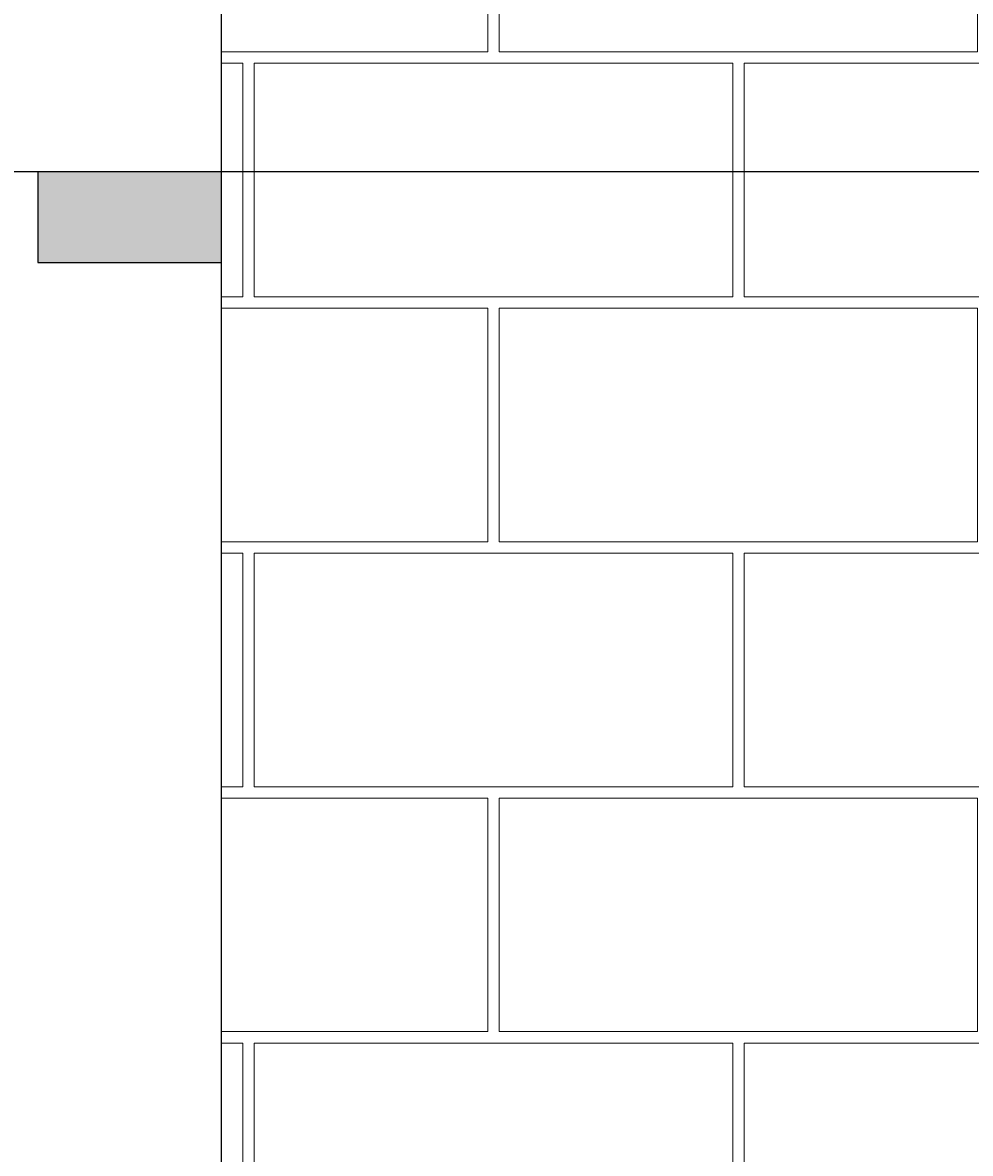
# Model space of a CAD drawing. Units: inches. Extents: x -128 to 854, y -395 to 398.
# Tile 54 of 61: x 405 to 467, y -322 to -248. Entities that reach past the tile are written whole.
import ezdxf

# ---------------------------------------------------------------- set-up
doc = ezdxf.new("R2010")
doc.units = ezdxf.units.IN
doc.header["$MEASUREMENT"] = 0
for name, color, linetype, lineweight in [('A-ANNO-DIMS', 2, 'Continuous', 18), ('A-ELEV', 3, 'Continuous', 25), ('A-ELEV-PATT', 8, 'Continuous', 13)]:
    doc.layers.add(name, color=color, linetype=linetype, lineweight=lineweight)
doc.styles.get("Standard").update_dxf_attribs({"font": 'arial.ttf'})
doc.dimstyles.get("Standard").update_dxf_attribs({"dimtxt": 0.18, "dimasz": 0.18, "dimexe": 0.18, "dimexo": 0.0625, "dimgap": 0.09, "dimtad": 0, "dimtih": 1, "dimtoh": 1, "dimdec": 1, "dimzin": 0, "dimdsep": 46, "dimlunit": 4, "dimtxsty": 'Standard', "dimcen": 0.09, "dimclrd": 1, "dimclre": 2, "dimclrt": 6, "dimadec": 0, "dimazin": 0, "dimtfac": 1, "dimtdec": 1, "dimtofl": 0, "dimtmove": 0, "dimatfit": 3, "dimfxl": 1, "dimtfill": 2, "dimtfillclr": 3, "dimtolj": 1, "dimtzin": 0, "dimarcsym": 0})

# ---------------------------------------------------------------- blocks, each defined once
blk = doc.blocks.new('*D134')
at = {"layer": 'A-ANNO-DIMS', "color": 2, "lineweight": -2, "transparency": 16777216}
for p, q in [((418.217, -191.476), (346.3, -191.476)), ((418.217, -371.476), (346.3, -371.476))]:
    blk.add_line(p, q, dxfattribs=at)
at = {"layer": 'A-ANNO-DIMS', "color": 1, "lineweight": -2, "transparency": 16777216}
for p, q in [((346.48, -191.656), (346.48, -281.295)), ((346.48, -371.296), (346.48, -281.658))]:
    blk.add_line(p, q, dxfattribs=at)
at = {"layer": 'A-ANNO-DIMS', "color": 1, "transparency": 16777216}
for points in [[(346.45, -191.656), (346.51, -191.656), (346.48, -191.476)], [(346.45, -371.296), (346.51, -371.296), (346.48, -371.476)]]:
    blk.add_solid(points, dxfattribs=at)
at = {"layer": 'Defpoints', "color": 0, "transparency": 16777216}
for p in [(346.48, -191.476), (418.28, -191.476), (418.28, -371.476)]:
    blk.add_point(p, dxfattribs=at)
at = {"layer": 'A-ANNO-DIMS', "color": 6, "transparency": 16777216, "insert": (346.48, -281.476), "char_height": 0.18, "attachment_point": 5, "bg_fill": 1, "box_fill_scale": 1.25, "bg_fill_color": 3, "bg_fill_transparency": 0}
blk.add_mtext('\\A1;15\'-0"', dxfattribs=at)
blk = doc.blocks.new('*D140')
at = {"layer": 'A-ANNO-DIMS', "color": 2, "lineweight": -2, "transparency": 16777216}
for p, q in [((551.245, -257.476), (346.3, -257.476)), ((551.245, -353.476), (346.3, -353.476))]:
    blk.add_line(p, q, dxfattribs=at)
at = {"layer": 'A-ANNO-DIMS', "color": 1, "lineweight": -2, "transparency": 16777216}
for p, q in [((346.48, -257.656), (346.48, -305.295)), ((346.48, -353.296), (346.48, -305.658))]:
    blk.add_line(p, q, dxfattribs=at)
at = {"layer": 'A-ANNO-DIMS', "color": 1, "transparency": 16777216}
for points in [[(346.45, -257.656), (346.51, -257.656), (346.48, -257.476)], [(346.45, -353.296), (346.51, -353.296), (346.48, -353.476)]]:
    blk.add_solid(points, dxfattribs=at)
at = {"layer": 'Defpoints', "color": 0, "transparency": 16777216}
for p in [(346.48, -257.476), (551.307, -257.476), (551.307, -353.476)]:
    blk.add_point(p, dxfattribs=at)
at = {"layer": 'A-ANNO-DIMS', "color": 6, "transparency": 16777216, "insert": (346.48, -305.476), "char_height": 0.18, "attachment_point": 5, "bg_fill": 1, "box_fill_scale": 1.25, "bg_fill_color": 3, "bg_fill_transparency": 0}
blk.add_mtext('\\A1;8\'-0"', dxfattribs=at)

msp = doc.modelspace()

# ---------------------------------------------------------------- hatches: boundary and pattern name
at = {"layer": 'A-ELEV-PATT'}
h = msp.add_hatch(dxfattribs=at)
h.set_pattern_fill('AR-B816C', color=256, scale=2)
h.set_pattern_definition([(0, (468.407, -10.41), (16, 16), [31.25, -0.75]), (0, (452.407, -9.66), (16, 16), [31.25, -0.75]), (90, (468.407, -10.41), (-16, 16), [-16.75, 15.25]), (90, (467.657, -10.41), (-16, 16), [-16.75, 15.25])])
h.paths.add_polyline_path([(418.28, -353.476), (492.252, -353.476), (492.252, -257.476), (551.307, -257.476), (551.307, -353.476), (782.28, -353.476), (782.28, -233.476), (418.28, -233.476)])
h.paths.add_polyline_path([(668.28, -257.476), (730.28, -257.476), (730.28, -305.476), (668.28, -305.476)], flags=16)
h.paths.add_polyline_path([(673.28, -300.476), (673.28, -262.476), (725.28, -262.476), (725.28, -300.476)], flags=0)
h = msp.add_hatch(color=256, dxfattribs=at)
h.dxf.hatch_style = 1
h.paths.add_polyline_path([(406.28, -257.476), (406.28, -258.401), (406.28, -263.401), (418.28, -263.401), (418.28, -257.476)])
h.paths.add_polyline_path([(794.28, -262.476), (794.28, -257.476), (782.28, -257.476), (782.28, -262.476)])

# ---------------------------------------------------------------- linework, layer by layer
at = {"layer": 'A-ELEV'}
for p, q in [((418.28, -257.476), (406.28, -257.476)), ((406.28, -257.476), (406.28, -258.401)), ((406.28, -258.401), (406.28, -263.401)), ((406.28, -263.401), (418.28, -263.401))]:
    msp.add_line(p, q, dxfattribs=at)
msp.add_lwpolyline([(418.28, -233.476), (782.28, -233.476), (782.28, -353.476), (418.28, -353.476)], close=True, dxfattribs=at)

# ---------------------------------------------------------------- dimensions: what is measured, and where the dimension line sits
at = {"layer": 'A-ANNO-DIMS'}
for base, p1, p2, picture, middle in [((346.48, -191.476), (418.28, -371.476), (418.28, -191.476), '*D134', (346.48, -281.476)), ((346.48, -257.476), (551.307, -353.476), (551.307, -257.476), '*D140', (346.48, -305.476))]:
    dim = msp.add_linear_dim(base=base, p1=p1, p2=p2, angle=90, dimstyle='Standard', override={"dimdec": 1, "dimlfac": 1, "dimrnd": 0, "dimzin": 1, "dimdsep": 46, "dimlunit": 4, "dimfrac": 2}, dxfattribs=at)
    dim.commit()
    dim.dimension.update_dxf_attribs({"geometry": picture, "text_midpoint": middle})

doc.saveas('drawing.dxf')
